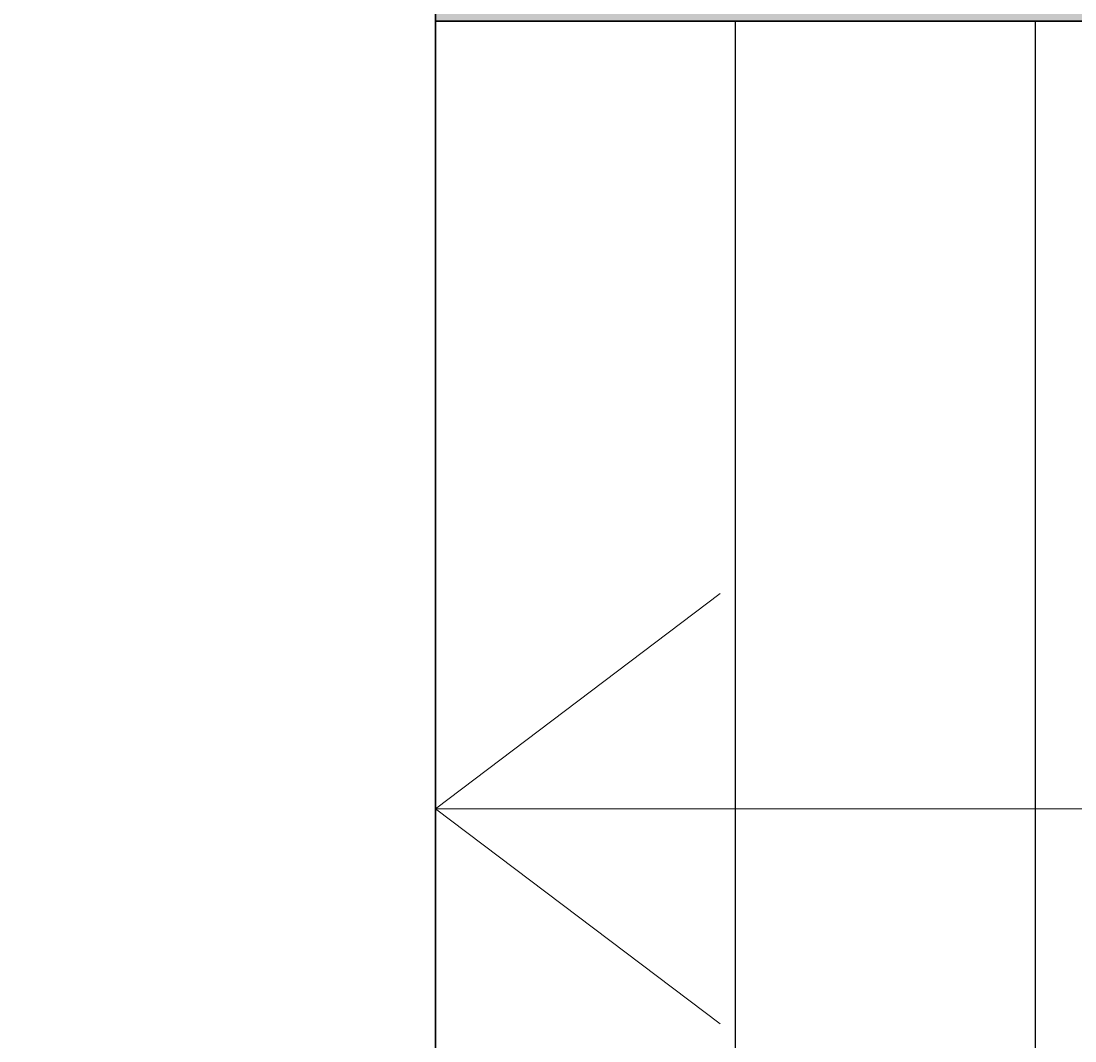
# Model space of a CAD drawing. Units: inches. Extents: x 1998 to 2588, y 1139 to 1977.
# Tile 88 of 134: x 2397 to 2425, y 1496 to 1523. Entities that reach past the tile are written whole.
import ezdxf

# ---------------------------------------------------------------- set-up
doc = ezdxf.new("R2010")
doc.units = ezdxf.units.IN
for name, color, linetype, lineweight in [('A-ANNO-DIMS', 2, 'Continuous', 18), ('A-ANNO-SYMB', 7, 'Continuous', 18), ('A-FLOR-EVTR', 7, 'Continuous', 35), ('A-FLOR-STRS', 7, 'Continuous', 25), ('A-WALL-PATT', 252, 'Continuous', 13)]:
    doc.layers.add(name, color=color, linetype=linetype, lineweight=lineweight)
doc.styles.get("Standard").update_dxf_attribs({"font": 'arial.ttf'})
doc.dimstyles.get("Standard").update_dxf_attribs({"dimtxt": 0.18, "dimasz": 0.18, "dimexe": 0.18, "dimexo": 0.0625, "dimgap": 0.09, "dimtad": 0, "dimtih": 1, "dimtoh": 1, "dimdec": 4, "dimzin": 0, "dimdsep": 46, "dimtxsty": 'Standard', "dimcen": 0.09, "dimadec": 0, "dimazin": 0, "dimtfac": 1, "dimtdec": 4, "dimtofl": 0, "dimtmove": 0, "dimatfit": 3, "dimfxl": 1, "dimtolj": 1, "dimtzin": 0, "dimarcsym": 0})

# ---------------------------------------------------------------- blocks, each defined once
blk = doc.blocks.new('*D24')
at = {"layer": 'A-ANNO-DIMS', "color": 0, "lineweight": -2, "transparency": 16777216}
for p, q in [((2398.535, 1911.232), (2588.309, 1911.232)), ((2588.129, 1911.052), (2588.129, 1570.164)), ((2588.129, 1228.912), (2588.129, 1569.8)), ((2527.535, 1228.732), (2588.309, 1228.732))]:
    blk.add_line(p, q, dxfattribs=at)
at = {"layer": 'A-ANNO-DIMS', "color": 0, "transparency": 16777216}
for points in [[(2588.099, 1911.052), (2588.159, 1911.052), (2588.129, 1911.232)], [(2588.099, 1228.912), (2588.159, 1228.912), (2588.129, 1228.732)]]:
    blk.add_solid(points, dxfattribs=at)
at = {"layer": 'Defpoints', "color": 0, "transparency": 16777216}
for p in [(2398.473, 1911.232), (2588.129, 1911.232), (2527.473, 1228.732)]:
    blk.add_point(p, dxfattribs=at)
at = {"layer": 'A-ANNO-DIMS', "color": 0, "transparency": 16777216, "insert": (2588.129, 1569.982), "char_height": 0.18, "attachment_point": 5}
blk.add_mtext('\\A1;682.5', dxfattribs=at)
blk = doc.blocks.new('*D43')
at = {"layer": 'A-ANNO-DIMS', "color": 0, "lineweight": -2, "transparency": 16777216}
for p, q in [((2407.973, 1594.67), (2407.973, 1138.602)), ((2345.973, 1588.67), (2345.973, 1138.602)), ((2346.153, 1138.782), (2376.754, 1138.782)), ((2407.793, 1138.782), (2377.191, 1138.782))]:
    blk.add_line(p, q, dxfattribs=at)
at = {"layer": 'A-ANNO-DIMS', "color": 0, "transparency": 16777216}
for points in [[(2346.153, 1138.812), (2346.153, 1138.752), (2345.973, 1138.782)], [(2407.793, 1138.812), (2407.793, 1138.752), (2407.973, 1138.782)]]:
    blk.add_solid(points, dxfattribs=at)
at = {"layer": 'Defpoints', "color": 0, "transparency": 16777216}
for p in [(2407.973, 1594.732), (2345.973, 1588.732), (2407.973, 1138.782)]:
    blk.add_point(p, dxfattribs=at)
at = {"layer": 'A-ANNO-DIMS', "color": 0, "transparency": 16777216, "insert": (2376.973, 1138.782), "char_height": 0.18, "attachment_point": 5}
blk.add_mtext('\\A1;62', dxfattribs=at)

msp = doc.modelspace()

# ---------------------------------------------------------------- hatches: boundary and pattern name
at = {"layer": 'A-WALL-PATT'}
h = msp.add_hatch(color=256, dxfattribs=at)
h.dxf.hatch_style = 1
h.paths.add_polyline_path([(2527.4729, 1362.2324), (2510.9729, 1362.2324), (2510.9729, 1357.7324), (2518.4729, 1357.7324), (2518.4729, 1237.7324), (2503.1458, 1237.7324), (2503.1458, 1228.7324), (2527.4729, 1228.7324)])
h.paths.add_polyline_path([(2490.5682, 1362.2324), (2398.4729, 1362.2324), (2398.4729, 1357.7324), (2490.5682, 1357.7324)])
h.paths.add_polyline_path([(2224.9729, 1264.7324), (2222.9729, 1264.7324), (2222.9729, 1232.4125), (2341.4729, 1232.4125), (2341.4729, 1234.4125), (2224.9729, 1234.4125)])
h.paths.add_polyline_path([(2334.5332, 1273.7324), (2264.7638, 1273.7324), (2264.7638, 1269.5611, -0.043659), (2264.3413, 1264.7324), (2334.5332, 1264.7324)])
h.paths.add_polyline_path([(2236.9551, 1273.7324), (2234.4125, 1273.7324), (2234.4125, 1264.7324), (2236.9551, 1264.7324), (2236.9551, 1269.5611)])
h.paths.add_polyline_path([(2222.9729, 1293.2324), (2096.9729, 1293.2324), (2096.9729, 1345.0966), (2087.9729, 1345.0966), (2087.9729, 1284.2324), (2222.9729, 1284.2324), (2222.9729, 1285.137)])
h.paths.add_polyline_path([(2096.9729, 1458.7927), (2087.9729, 1458.7927), (2087.9729, 1417.7324), (2087.9729, 1413.2324), (2096.9729, 1413.2324), (2096.9729, 1417.7324)])
h.paths.add_polyline_path([(2096.9729, 1413.2324), (2087.9729, 1413.2324), (2087.9729, 1365.5012), (2096.9729, 1365.5012), (2096.9729, 1369.3358)])
h.paths.add_polyline_path([(2186.2943, 1417.7324), (2138.6074, 1417.7324), (2096.9729, 1417.7324), (2096.9729, 1413.2324), (2138.6074, 1413.2324), (2186.2943, 1413.2324)])
h.paths.add_polyline_path([(2181.4729, 1465.7324), (2176.9729, 1465.7324), (2176.9729, 1451.6434), (2181.4729, 1451.6434)])
h.paths.add_polyline_path([(2181.4729, 1422.1664), (2176.9729, 1422.1664), (2176.9729, 1417.7324), (2181.4729, 1417.7324)])
h.paths.add_polyline_path([(2063.9729, 1465.7324), (2087.9729, 1465.7324), (2087.9729, 1470.2324), (2059.4729, 1470.2324), (2059.4729, 1413.2324), (2087.9729, 1413.2324), (2087.9729, 1417.7324), (2063.9729, 1417.7324)])
h.paths.add_polyline_path([(2181.4729, 1755.2324), (2176.9729, 1755.2324), (2176.9729, 1748.6798), (2177.0513, 1748.6798), (2181.4729, 1748.6798)])
h.paths.add_polyline_path([(2227.4729, 1707.2324), (2220.4647, 1707.2324), (2220.4647, 1702.7324), (2222.9729, 1702.7324), (2222.9729, 1604.637), (2227.4729, 1604.637)])
h.paths.add_polyline_path([(2114.9729, 1702.7324), (2105.9729, 1702.7324), (2105.9729, 1628.4781, -0.0318759), (2110.1012, 1628.7416), (2114.9729, 1628.7416)])
h.paths.add_polyline_path([(2345.9729, 1739.3278), (2341.4729, 1739.3278), (2341.4729, 1647.5211), (2345.9729, 1647.5211)])
h.paths.add_polyline_path([(2350.6273, 1641.2324), (2345.9729, 1641.2324), (2345.9729, 1636.7324), (2350.6273, 1636.7324), (2350.6273, 1639.8729)])
h.paths.add_polyline_path([(2501.9729, 1641.2324), (2407.9729, 1641.2324), (2392.5005, 1641.2324), (2392.5005, 1639.8729), (2392.5005, 1636.7324), (2501.9729, 1636.7324)])
h.paths.add_polyline_path([(2510.9729, 1755.2324), (2501.9729, 1755.2324), (2501.9729, 1641.2324), (2510.9729, 1641.2324)])
h.paths.add_polyline_path([(2549.1786, 1641.2324), (2522.3775, 1641.2324), (2522.3775, 1636.7324), (2540.1786, 1636.7324), (2540.1786, 1480.7324), (2522.3775, 1480.7324), (2522.3775, 1476.2324), (2549.1786, 1476.2324)])
h.paths.add_polyline_path([(2498.1786, 1594.7324), (2407.9729, 1594.7324), (2407.9729, 1585.7324), (2416.9729, 1585.7324), (2489.1786, 1585.7324), (2489.1786, 1531.7324), (2416.9729, 1531.7324), (2407.9729, 1531.7324), (2407.9729, 1522.7324), (2498.1786, 1522.7324)])
h.paths.add_polyline_path([(2351.6437, 1480.7324), (2345.9729, 1480.7324), (2345.9729, 1476.2324), (2351.6437, 1476.2324), (2351.6437, 1477.5919)])
h.paths.add_polyline_path([(2501.9729, 1480.7324), (2498.1786, 1480.7324), (2407.9729, 1480.7324), (2393.5168, 1480.7324), (2393.5168, 1477.5919), (2393.5168, 1476.2324), (2501.9729, 1476.2324)])

# ---------------------------------------------------------------- linework, layer by layer
at = {"layer": 'A-ANNO-SYMB'}
for q in [(2415.5619, 1507.4684), (2498.1786, 1501.7324), (2415.5619, 1495.9963)]:
    msp.add_line((2407.9729, 1501.7324), q, dxfattribs=at)
at = {"layer": 'A-FLOR-EVTR'}
msp.add_lwpolyline([(2407.9729, 1522.7324), (2498.1786, 1522.7324), (2498.1786, 1594.7324), (2407.9729, 1594.7324)], close=True, dxfattribs=at)
at = {"layer": 'A-FLOR-STRS'}
for p, q in [((2407.9729, 1480.7324), (2407.9729, 1636.7324)), ((2540.1786, 1522.7324), (2407.9729, 1522.7324)), ((2407.9729, 1480.7324), (2407.9729, 1522.7324)), ((2415.9729, 1480.7324), (2415.9729, 1522.7324)), ((2423.9729, 1480.7324), (2423.9729, 1522.7324))]:
    msp.add_line(p, q, dxfattribs=at)

# ---------------------------------------------------------------- dimensions: what is measured, and where the dimension line sits
at = {"layer": 'A-ANNO-DIMS'}
dim = msp.add_linear_dim(base=(2588.1286, 1911.2324), p1=(2527.4729, 1228.7324), p2=(2398.4729, 1911.2324), angle=90, dimstyle='Standard', override={"dimdec": 1, "dimlfac": 1, "dimrnd": 0, "dimzin": 0, "dimdsep": 46, "dimlunit": 2}, dxfattribs=at)
dim.commit()
dim.dimension.update_dxf_attribs({"geometry": '*D24', "text_midpoint": (2588.1286, 1569.9824)})
dim = msp.add_linear_dim(base=(2407.9729, 1138.7824), p1=(2345.9729, 1588.7324), p2=(2407.9729, 1594.7324), dimstyle='Standard', override={"dimdec": 0, "dimlfac": 1, "dimrnd": 0, "dimzin": 0, "dimdsep": 46, "dimlunit": 2}, dxfattribs=at)
dim.commit()
dim.dimension.update_dxf_attribs({"geometry": '*D43', "text_midpoint": (2376.9729, 1138.7824)})

doc.saveas('drawing.dxf')
